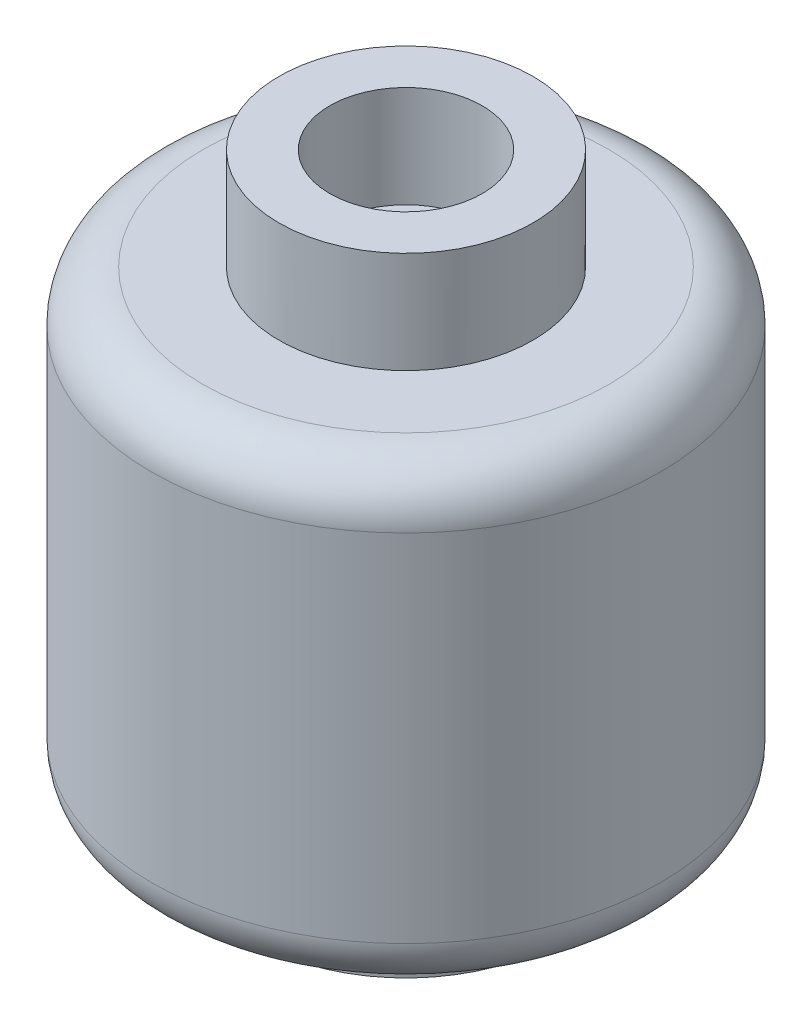
ISO-10303-21;
HEADER;
FILE_DESCRIPTION(('STEP AP214'),'2;1');
FILE_NAME('part.step','',(''),(''),'','','');
FILE_SCHEMA(('AUTOMOTIVE_DESIGN { 1 0 10303 214 1 1 1 1 }'));
ENDSEC;
DATA;
#1=APPLICATION_CONTEXT('core data for automotive mechanical design processes');
#2=APPLICATION_PROTOCOL_DEFINITION('international standard','automotive_design',2000,#1);
#3=PRODUCT_CONTEXT('',#1,'mechanical');
#4=PRODUCT('Part','Part','',(#3));
#5=PRODUCT_RELATED_PRODUCT_CATEGORY('part','',(#4));
#6=PRODUCT_DEFINITION_FORMATION('','',#4);
#7=PRODUCT_DEFINITION_CONTEXT('part definition',#1,'design');
#8=PRODUCT_DEFINITION('design','',#6,#7);
#9=PRODUCT_DEFINITION_SHAPE('','',#8);
#10=(LENGTH_UNIT() NAMED_UNIT(*) SI_UNIT(.MILLI.,.METRE.));
#11=(NAMED_UNIT(*) PLANE_ANGLE_UNIT() SI_UNIT($,.RADIAN.));
#12=(NAMED_UNIT(*) SI_UNIT($,.STERADIAN.) SOLID_ANGLE_UNIT());
#13=UNCERTAINTY_MEASURE_WITH_UNIT(LENGTH_MEASURE(1.E-05),#10,'distance_accuracy_value','');
#14=(GEOMETRIC_REPRESENTATION_CONTEXT(3) GLOBAL_UNCERTAINTY_ASSIGNED_CONTEXT((#13)) GLOBAL_UNIT_ASSIGNED_CONTEXT((#10,
#11,#12)) REPRESENTATION_CONTEXT('',''));
#15=CARTESIAN_POINT('',(0.,0.,0.));
#16=DIRECTION('',(0.,0.,1.));
#17=DIRECTION('',(1.,0.,0.));
#18=AXIS2_PLACEMENT_3D('',#15,#16,#17);
#19=CARTESIAN_POINT('',(0.,0.,0.));
#20=DIRECTION('',(0.,-1.,0.));
#21=DIRECTION('',(0.,0.,-1.));
#22=AXIS2_PLACEMENT_3D('',#19,#20,#21);
#23=CYLINDRICAL_SURFACE('',#22,5.);
#24=CARTESIAN_POINT('',(1.,6.20000000000001,-4.89897948556635));
#25=CARTESIAN_POINT('',(1.00000156872369,6.23586306138393,-4.89897950578697));
#26=CARTESIAN_POINT('',(1.00297865499742,6.27174942589603,-4.89837438780102));
#27=CARTESIAN_POINT('',(1.01480213788461,6.34252588569872,-4.89593828236374));
#28=CARTESIAN_POINT('',(1.02365483576842,6.37741486940713,-4.89410597880414));
#29=CARTESIAN_POINT('',(1.04694279696722,6.44516035531958,-4.88917697960863));
#30=CARTESIAN_POINT('',(1.06137459390475,6.47801810488525,-4.88608106900412));
#31=CARTESIAN_POINT('',(1.09535369815749,6.54079511555044,-4.87857576446154));
#32=CARTESIAN_POINT('',(1.11489983070227,6.57071504930283,-4.87416667213113));
#33=CARTESIAN_POINT('',(1.158584541537,6.62694759387382,-4.86396809819116));
#34=CARTESIAN_POINT('',(1.18274402944443,6.65324280362197,-4.8581722999757));
#35=CARTESIAN_POINT('',(1.23482548770339,6.70138615204387,-4.84519606525274));
#36=CARTESIAN_POINT('',(1.26274776156696,6.72323393162384,-4.83801551702904));
#37=CARTESIAN_POINT('',(1.3220159987903,6.76232468706743,-4.82216028574895));
#38=CARTESIAN_POINT('',(1.35341419297984,6.77947847351074,-4.81346121280438));
#39=CARTESIAN_POINT('',(1.41825919170025,6.80832243059168,-4.79475540886427));
#40=CARTESIAN_POINT('',(1.45170630441394,6.8200117770161,-4.78474848089322));
#41=CARTESIAN_POINT('',(1.52093621337638,6.83809739450905,-4.76320407601995));
#42=CARTESIAN_POINT('',(1.55675973455566,6.84428700126766,-4.75162434130285));
#43=CARTESIAN_POINT('',(1.6286066450515,6.85064895607429,-4.72748115596413));
#44=CARTESIAN_POINT('',(1.66463008196061,6.85081980390408,-4.71491746086553));
#45=CARTESIAN_POINT('',(1.73778614615725,6.8451409167464,-4.68846317663509));
#46=CARTESIAN_POINT('',(1.77488244422993,6.83898557672516,-4.67453760951146));
#47=CARTESIAN_POINT('',(1.84736298119408,6.82044202595814,-4.64637104142785));
#48=CARTESIAN_POINT('',(1.88274670164537,6.808051940576,-4.63212994682831));
#49=CARTESIAN_POINT('',(1.95230180183688,6.7767372104701,-4.60325879116952));
#50=CARTESIAN_POINT('',(1.9863675791089,6.75757032988729,-4.58863604916084));
#51=CARTESIAN_POINT('',(2.05076153491668,6.71324275804796,-4.56022117549695));
#52=CARTESIAN_POINT('',(2.08108914696987,6.68808116004063,-4.54642916989329));
#53=CARTESIAN_POINT('',(2.13666734384406,6.63263773864959,-4.52057310799027));
#54=CARTESIAN_POINT('',(2.16197848776713,6.60242630418322,-4.50848902040552));
#55=CARTESIAN_POINT('',(2.20700707163729,6.53735060646704,-4.48661882658691));
#56=CARTESIAN_POINT('',(2.22672828488387,6.50248950530907,-4.47683117099428));
#57=CARTESIAN_POINT('',(2.25819322579238,6.43227479843316,-4.46103664936299));
#58=CARTESIAN_POINT('',(2.27047667241963,6.39722069281157,-4.45477724754247));
#59=CARTESIAN_POINT('',(2.28891940690895,6.32514791726527,-4.44532990950916));
#60=CARTESIAN_POINT('',(2.29508397912362,6.28813097163815,-4.44213932309484));
#61=CARTESIAN_POINT('',(2.30064016771881,6.21728843643163,-4.43926371696131));
#62=CARTESIAN_POINT('',(2.30066024102716,6.18352384179948,-4.43925341767421));
#63=CARTESIAN_POINT('',(2.29549044487861,6.11650916532808,-4.44192887306966));
#64=CARTESIAN_POINT('',(2.29030144628595,6.08325899842914,-4.44461417709524));
#65=CARTESIAN_POINT('',(2.2751970896081,6.01922729119317,-4.4523641461491));
#66=CARTESIAN_POINT('',(2.26542901508946,5.98840154076483,-4.45735459869809));
#67=CARTESIAN_POINT('',(2.2416246503813,5.92887550666932,-4.4693730916337));
#68=CARTESIAN_POINT('',(2.22758750274041,5.90017565143361,-4.47640154134266));
#69=CARTESIAN_POINT('',(2.19475446312109,5.84381199746009,-4.49259464275087));
#70=CARTESIAN_POINT('',(2.17572169113451,5.81631645313862,-4.50186295811208));
#71=CARTESIAN_POINT('',(2.13398524683761,5.76484784883829,-4.52179628349611));
#72=CARTESIAN_POINT('',(2.11128006898282,5.74087624126394,-4.53246186600219));
#73=CARTESIAN_POINT('',(2.0603132664187,5.69458448372974,-4.55587219554798));
#74=CARTESIAN_POINT('',(2.03172164052999,5.67267848035175,-4.56871810401778));
#75=CARTESIAN_POINT('',(1.97152502592908,5.63395784409478,-4.59501563982341));
#76=CARTESIAN_POINT('',(1.93991878964557,5.61714533123995,-4.60846751670828));
#77=CARTESIAN_POINT('',(1.87189090526185,5.58784074539247,-4.63653729284295));
#78=CARTESIAN_POINT('',(1.83528586966668,5.57578175770425,-4.65116512383152));
#79=CARTESIAN_POINT('',(1.76037210083443,5.55828524067232,-4.68003221408688));
#80=CARTESIAN_POINT('',(1.72206312404718,5.55284866106503,-4.69427141733338));
#81=CARTESIAN_POINT('',(1.64430475631013,5.54884647842725,-4.72207434484025));
#82=CARTESIAN_POINT('',(1.60484715620024,5.55036544303433,-4.7356277187452));
#83=CARTESIAN_POINT('',(1.52645695557744,5.56062652830447,-4.76147365799019));
#84=CARTESIAN_POINT('',(1.48752423425738,5.5693669569861,-4.773766517909));
#85=CARTESIAN_POINT('',(1.41306705492273,5.59350921700795,-4.79632087238086));
#86=CARTESIAN_POINT('',(1.37746829085197,5.60862278292357,-4.80664505170919));
#87=CARTESIAN_POINT('',(1.30919735599651,5.64515691876416,-4.82568736070702));
#88=CARTESIAN_POINT('',(1.27652417332082,5.66657529692486,-4.83440604679051));
#89=CARTESIAN_POINT('',(1.2168920567295,5.71390195966075,-4.84974997525069));
#90=CARTESIAN_POINT('',(1.18972498577156,5.73952074592783,-4.85646016611695));
#91=CARTESIAN_POINT('',(1.14003765055289,5.79523971609589,-4.86836405127563));
#92=CARTESIAN_POINT('',(1.11751752335932,5.82534003213987,-4.87355770083774));
#93=CARTESIAN_POINT('',(1.07859052667666,5.88805669287335,-4.88231795370564));
#94=CARTESIAN_POINT('',(1.06200451295069,5.92055534099506,-4.88593312985496));
#95=CARTESIAN_POINT('',(1.0344876911731,5.98794797415707,-4.89183350906889));
#96=CARTESIAN_POINT('',(1.023550119189,6.02283903730369,-4.89412030326468));
#97=CARTESIAN_POINT('',(1.01042863815805,6.08161266137401,-4.89684186503736));
#98=CARTESIAN_POINT('',(1.00652375664101,6.10510902941916,-4.89764403406034));
#99=CARTESIAN_POINT('',(1.00130892684902,6.1524001773894,-4.89871283556499));
#100=CARTESIAN_POINT('',(0.999998958718624,6.17619495502974,-4.8989794721444));
#101=CARTESIAN_POINT('',(1.,6.20000000000001,-4.89897948556635));
#102=B_SPLINE_CURVE_WITH_KNOTS('',3,(#24,#25,#26,#27,#28,#29,#30,#31,#32,#33,#34,#35,#36,#37,
#38,#39,#40,#41,#42,#43,#44,#45,#46,#47,#48,#49,#50,#51,#52,#53,#54,#55,#56,#57,#58,#59,#60,#61,
#62,#63,#64,#65,#66,#67,#68,#69,#70,#71,#72,#73,#74,#75,#76,#77,#78,#79,#80,#81,#82,#83,#84,#85,
#86,#87,#88,#89,#90,#91,#92,#93,#94,#95,#96,#97,#98,#99,#100,#101),.UNSPECIFIED.,.T.,.F.,(4,2,2,
2,2,2,2,2,2,2,2,2,2,2,2,2,2,2,2,2,2,2,2,2,2,2,2,2,2,2,2,2,2,2,2,2,2,2,4),(0.,0.107502146017198,
0.215119768867601,0.322670634469891,0.43019681713439,0.538222445139969,0.6462567918788,
0.756220203332003,0.866200195455233,0.980156747892354,1.09414170460534,1.21390423220609,
1.33370279102324,1.45830794042833,1.58293194937669,1.70594505008929,1.82887491601095,
1.94124585538271,2.05351966485334,2.15430587581719,2.25507523992364,2.3528050697022,
2.45055454167926,2.55422921628436,2.65794650173261,2.77218412218085,2.88646922575167,
3.00956635425307,3.13268113435011,3.25729672894529,3.38188313451486,3.50135381061271,
3.6207830036443,3.73403554896939,3.84729143433638,3.95676250922337,4.06610218822255,
4.1374600953053,4.20881745637782),.UNSPECIFIED.);
#103=CARTESIAN_POINT('',(1.,6.20000000000001,-4.89897948556635));
#104=VERTEX_POINT('',#103);
#105=EDGE_CURVE('E74',#104,#104,#102,.T.);
#106=ORIENTED_EDGE('',*,*,#105,.F.);
#107=EDGE_LOOP('',(#106));
#108=FACE_BOUND('',#107,.T.);
#109=CARTESIAN_POINT('',(-2.3,6.2,-4.43959457608462));
#110=CARTESIAN_POINT('',(-2.29999812506802,6.23376367901104,-4.43959590662005));
#111=CARTESIAN_POINT('',(-2.29735527963792,6.26755114267601,-4.44096780412534));
#112=CARTESIAN_POINT('',(-2.28690648695137,6.3341211679552,-4.44635710752491));
#113=CARTESIAN_POINT('',(-2.27909442133407,6.36690249051653,-4.45037764836535));
#114=CARTESIAN_POINT('',(-2.25869913357096,6.43042247308173,-4.46076311262972));
#115=CARTESIAN_POINT('',(-2.24613138854528,6.46116738310239,-4.46712042923328));
#116=CARTESIAN_POINT('',(-2.21672094698416,6.52001627619411,-4.48178727121732));
#117=CARTESIAN_POINT('',(-2.19987807861373,6.54812015304884,-4.49009687506733));
#118=CARTESIAN_POINT('',(-2.16146430546663,6.60258307597295,-4.50871936393883));
#119=CARTESIAN_POINT('',(-2.13968914881422,6.62876912685022,-4.51911545385904));
#120=CARTESIAN_POINT('',(-2.09263608544451,6.6771942600584,-4.54109553218148));
#121=CARTESIAN_POINT('',(-2.06735681864845,6.69943180214097,-4.5526799813752));
#122=CARTESIAN_POINT('',(-2.01117236237794,6.74167522592829,-4.57779690806998));
#123=CARTESIAN_POINT('',(-1.97995632831079,6.76122203264447,-4.59140755455667));
#124=CARTESIAN_POINT('',(-1.91479516687287,6.79474970564269,-4.6189621878202));
#125=CARTESIAN_POINT('',(-1.8808489780272,6.80872839436278,-4.63290630275346));
#126=CARTESIAN_POINT('',(-1.80891617263393,6.83146833025578,-4.66148114234036));
#127=CARTESIAN_POINT('',(-1.77080935365711,6.83986364832348,-4.67610249687003));
#128=CARTESIAN_POINT('',(-1.69345543478325,6.84971654668912,-4.70466876542849));
#129=CARTESIAN_POINT('',(-1.65420831894334,6.85117402993979,-4.71861366999231));
#130=CARTESIAN_POINT('',(-1.57597436565614,6.84694985361812,-4.74531362816683));
#131=CARTESIAN_POINT('',(-1.53698753163237,6.84131556866086,-4.75807597249634));
#132=CARTESIAN_POINT('',(-1.46026544439222,6.82294082952768,-4.78217950617192));
#133=CARTESIAN_POINT('',(-1.42252982962489,6.81020244744065,-4.79352110873239));
#134=CARTESIAN_POINT('',(-1.35141826472214,6.77860919080583,-4.81403920055205));
#135=CARTESIAN_POINT('',(-1.3179195617974,6.76008169831667,-4.8232941306707));
#136=CARTESIAN_POINT('',(-1.25443098431052,6.71719555150431,-4.84019450796681));
#137=CARTESIAN_POINT('',(-1.22444010474567,6.69283857346974,-4.84784041663832));
#138=CARTESIAN_POINT('',(-1.1703996413989,6.64026821999595,-4.86116283805444));
#139=CARTESIAN_POINT('',(-1.14613384708423,6.61229632782405,-4.86691631700377));
#140=CARTESIAN_POINT('',(-1.10260925091337,6.55246437083802,-4.87696147784919));
#141=CARTESIAN_POINT('',(-1.08334962935697,6.5206049438176,-4.8812533990934));
#142=CARTESIAN_POINT('',(-1.05095875369573,6.45486363174064,-4.88832836599271));
#143=CARTESIAN_POINT('',(-1.03767282381066,6.42106198815578,-4.89114983844069));
#144=CARTESIAN_POINT('',(-1.0168991773021,6.35164312266193,-4.89551118022622));
#145=CARTESIAN_POINT('',(-1.00941105205768,6.31602602889187,-4.89705113988351));
#146=CARTESIAN_POINT('',(-1.00052599399766,6.24440378746397,-4.89887418995811));
#147=CARTESIAN_POINT('',(-0.999063698312998,6.20840707349181,-4.89917076809482));
#148=CARTESIAN_POINT('',(-1.00209674620955,6.13667654340366,-4.89855125681151));
#149=CARTESIAN_POINT('',(-1.00659192846425,6.10094272019503,-4.89763520022925));
#150=CARTESIAN_POINT('',(-1.02137894203311,6.03083740653594,-4.89457262804262));
#151=CARTESIAN_POINT('',(-1.03165734384401,5.99646295663634,-4.89242896292495));
#152=CARTESIAN_POINT('',(-1.0576725461085,5.92995718247656,-4.88687063433681));
#153=CARTESIAN_POINT('',(-1.07340928449704,5.89782583271577,-4.88345598531827));
#154=CARTESIAN_POINT('',(-1.10989933958094,5.83659142641726,-4.87529206174308));
#155=CARTESIAN_POINT('',(-1.13066931077326,5.80749889214164,-4.87053834768339));
#156=CARTESIAN_POINT('',(-1.17653144201685,5.75324569098518,-4.85966332997484));
#157=CARTESIAN_POINT('',(-1.20162370731765,5.72808511987762,-4.85354199302276));
#158=CARTESIAN_POINT('',(-1.25567798189552,5.68203622483806,-4.83984072339389));
#159=CARTESIAN_POINT('',(-1.28468462187544,5.66120550696568,-4.8322434424138));
#160=CARTESIAN_POINT('',(-1.34541503278201,5.62468788796898,-4.81568772478889));
#161=CARTESIAN_POINT('',(-1.37713909767426,5.6090015442413,-4.80672914079969));
#162=CARTESIAN_POINT('',(-1.44331517189571,5.58267858194895,-4.78728141776184));
#163=CARTESIAN_POINT('',(-1.47781951323458,5.57220093972653,-4.7767555385319));
#164=CARTESIAN_POINT('',(-1.54772794803604,5.55710011700076,-4.75456454632537));
#165=CARTESIAN_POINT('',(-1.58313224008343,5.55247824028405,-4.74289918026448));
#166=CARTESIAN_POINT('',(-1.65557732195721,5.54896631995416,-4.71811362760663));
#167=CARTESIAN_POINT('',(-1.6926170146506,5.5503551676754,-4.70495087491527));
#168=CARTESIAN_POINT('',(-1.76571140828362,5.55932234894575,-4.67801051902459));
#169=CARTESIAN_POINT('',(-1.80176582787881,5.56690243170286,-4.66423274310303));
#170=CARTESIAN_POINT('',(-1.87372731403228,5.58850604851756,-4.63580776547661));
#171=CARTESIAN_POINT('',(-1.90954229589548,5.60282446177242,-4.62115082194428));
#172=CARTESIAN_POINT('',(-1.97820531554219,5.63762702889237,-4.59217748603411));
#173=CARTESIAN_POINT('',(-2.01105262354813,5.65811269400359,-4.57786117805572));
#174=CARTESIAN_POINT('',(-2.0732244717038,5.7051088127454,-4.55004552514963));
#175=CARTESIAN_POINT('',(-2.10250284820064,5.73168753395944,-4.53655781952078));
#176=CARTESIAN_POINT('',(-2.1560901046185,5.79018972336251,-4.51133619308962));
#177=CARTESIAN_POINT('',(-2.18039937266147,5.82211277376767,-4.49960213533447));
#178=CARTESIAN_POINT('',(-2.22172826438218,5.88845238309648,-4.4793328811199));
#179=CARTESIAN_POINT('',(-2.2390976859563,5.92260450599742,-4.47064802319505));
#180=CARTESIAN_POINT('',(-2.26766152055505,5.99393686274579,-4.45622833058083));
#181=CARTESIAN_POINT('',(-2.27887023211448,6.03110985303888,-4.45048666706987));
#182=CARTESIAN_POINT('',(-2.29109776124512,6.09056742051539,-4.44419773201944));
#183=CARTESIAN_POINT('',(-2.29442856701929,6.11228002584481,-4.44247720641403));
#184=CARTESIAN_POINT('',(-2.29888023963348,6.15599172862197,-4.44017522460793));
#185=CARTESIAN_POINT('',(-2.300001222193,6.17799081100734,-4.43959370876191));
#186=CARTESIAN_POINT('',(-2.3,6.2,-4.43959457608462));
#187=B_SPLINE_CURVE_WITH_KNOTS('',3,(#109,#110,#111,#112,#113,#114,#115,#116,#117,#118,#119,
#120,#121,#122,#123,#124,#125,#126,#127,#128,#129,#130,#131,#132,#133,#134,#135,#136,#137,#138,
#139,#140,#141,#142,#143,#144,#145,#146,#147,#148,#149,#150,#151,#152,#153,#154,#155,#156,#157,
#158,#159,#160,#161,#162,#163,#164,#165,#166,#167,#168,#169,#170,#171,#172,#173,#174,#175,#176,
#177,#178,#179,#180,#181,#182,#183,#184,#185,#186),.UNSPECIFIED.,.T.,.F.,(4,2,2,2,2,2,2,2,2,2,2,
2,2,2,2,2,2,2,2,2,2,2,2,2,2,2,2,2,2,2,2,2,2,2,2,2,2,2,4),(0.,0.101204556162369,
0.202529114228452,0.303526713773192,0.40452837347427,0.510916737967762,0.617346512073878,
0.734633479254858,0.851966269723879,0.976382548008533,1.10080056663807,1.22439183858376,
1.34794708086105,1.46549698438377,1.58301312655323,1.69488360571627,1.80673575588673,
1.9154962801722,2.0242491384745,2.13181918581453,2.23938632025301,2.34670469249778,
2.45402184449863,2.56169906761254,2.66937891307903,2.77841072259549,2.8874543418872,
2.99964818476995,3.11186700323271,3.22934710116267,3.34686040219996,3.47007725828108,
3.59332433248496,3.71802633388025,3.84271859145621,3.95993123548691,4.07687067669987,
4.1428453251822,4.20881651874698),.UNSPECIFIED.);
#188=CARTESIAN_POINT('',(-2.3,6.2,-4.43959457608462));
#189=VERTEX_POINT('',#188);
#190=EDGE_CURVE('E84',#189,#189,#187,.T.);
#191=ORIENTED_EDGE('',*,*,#190,.F.);
#192=EDGE_LOOP('',(#191));
#193=FACE_BOUND('',#192,.T.);
#194=CARTESIAN_POINT('',(0.,8.99999999999999,0.));
#195=DIRECTION('',(0.,-1.,0.));
#196=DIRECTION('',(0.,0.,-1.));
#197=AXIS2_PLACEMENT_3D('',#194,#195,#196);
#198=CIRCLE('',#197,5.);
#199=CARTESIAN_POINT('',(0.,8.99999999999999,-5.));
#200=VERTEX_POINT('',#199);
#201=EDGE_CURVE('E141',#200,#200,#198,.T.);
#202=ORIENTED_EDGE('',*,*,#201,.T.);
#203=EDGE_LOOP('',(#202));
#204=FACE_BOUND('',#203,.T.);
#205=CARTESIAN_POINT('',(0.,2.00000000000001,0.));
#206=DIRECTION('',(0.,-1.,0.));
#207=DIRECTION('',(0.,0.,-1.));
#208=AXIS2_PLACEMENT_3D('',#205,#206,#207);
#209=CIRCLE('',#208,5.);
#210=CARTESIAN_POINT('',(0.,2.00000000000001,-5.));
#211=VERTEX_POINT('',#210);
#212=EDGE_CURVE('E149',#211,#211,#209,.T.);
#213=ORIENTED_EDGE('',*,*,#212,.F.);
#214=EDGE_LOOP('',(#213));
#215=FACE_BOUND('',#214,.T.);
#216=CARTESIAN_POINT('',(-2.1920310216783,3.30796897832171,-4.49388473372426));
#217=CARTESIAN_POINT('',(-2.19203989382054,3.31536049313591,-4.49387988155964));
#218=CARTESIAN_POINT('',(-2.19145216951387,3.32274502445388,-4.49416708637392));
#219=CARTESIAN_POINT('',(-2.1891546068307,3.33726856084877,-4.49528697229227));
#220=CARTESIAN_POINT('',(-2.18744882171491,3.34440835514677,-4.49611768302666));
#221=CARTESIAN_POINT('',(-2.18298660118061,3.35826307582907,-4.49828581107898));
#222=CARTESIAN_POINT('',(-2.18023077750409,3.36497824694372,-4.49962293336386));
#223=CARTESIAN_POINT('',(-2.17378026863328,3.37783109618784,-4.50274274527229));
#224=CARTESIAN_POINT('',(-2.17008498152936,3.38396840061333,-4.50452572053962));
#225=CARTESIAN_POINT('',(-2.16171016813163,3.39578311874742,-4.50855093565586));
#226=CARTESIAN_POINT('',(-2.15699559881476,3.40143006609363,-4.51080942207691));
#227=CARTESIAN_POINT('',(-2.14683728896301,3.4118597250654,-4.51565292338937));
#228=CARTESIAN_POINT('',(-2.14139334787007,3.41664219813053,-4.51823802808103));
#229=CARTESIAN_POINT('',(-2.1293736528847,3.42568934690085,-4.52391600578119));
#230=CARTESIAN_POINT('',(-2.12273944414948,3.42986069087341,-4.52703379636494));
#231=CARTESIAN_POINT('',(-2.10895287896103,3.43702905069902,-4.5334728165519));
#232=CARTESIAN_POINT('',(-2.10180022246091,3.44002537998886,-4.53679416378711));
#233=CARTESIAN_POINT('',(-2.08737980857593,3.44473030946788,-4.54344651338));
#234=CARTESIAN_POINT('',(-2.08012242134716,3.44647580810284,-4.54677405226762));
#235=CARTESIAN_POINT('',(-2.06544925264667,3.44880578897676,-4.55345866408099));
#236=CARTESIAN_POINT('',(-2.05803370616546,3.44939188683814,-4.55681568935138));
#237=CARTESIAN_POINT('',(-2.05060966544099,3.44939033455901,-4.56015350618814));
#238=B_SPLINE_CURVE_WITH_KNOTS('',3,(#216,#217,#218,#219,#220,#221,#222,#223,#224,#225,#226,
#227,#228,#229,#230,#231,#232,#233,#234,#235,#236,#237),.UNSPECIFIED.,.F.,.F.,(4,2,2,2,2,2,2,2,
2,2,4),(0.,0.0221347353454418,0.0441896670813337,0.0662317694314662,0.0882880297959428,
0.111277980951727,0.134274266763733,0.159470948812198,0.184682331468863,0.209115401679695,
0.233514400409308),.UNSPECIFIED.);
#239=CARTESIAN_POINT('',(-2.1920310216783,3.30796897832171,-4.49388473372426));
#240=VERTEX_POINT('',#239);
#241=CARTESIAN_POINT('',(-2.05060966544099,3.44939033455901,-4.56015350618814));
#242=VERTEX_POINT('',#241);
#243=EDGE_CURVE('E11',#240,#242,#238,.T.);
#244=ORIENTED_EDGE('',*,*,#243,.F.);
#245=CARTESIAN_POINT('',(2.1920310216783,3.3079689783217,-4.49388473372426));
#246=CARTESIAN_POINT('',(2.1329852864635,3.24894496168585,-4.52268309678667));
#247=CARTESIAN_POINT('',(2.07154515480206,3.1922576989043,-4.55121205387414));
#248=CARTESIAN_POINT('',(1.94394561125621,3.0837785042517,-4.60716301673319));
#249=CARTESIAN_POINT('',(1.87778329480569,3.03198963166128,-4.63458432467978));
#250=CARTESIAN_POINT('',(1.67169372276185,2.88387898486698,-4.71456634831918));
#251=CARTESIAN_POINT('',(1.52480314791688,2.79545604567751,-4.76452160426455));
#252=CARTESIAN_POINT('',(1.2927352314236,2.68107152816368,-4.83067294967581));
#253=CARTESIAN_POINT('',(1.21318555917039,2.64591269927123,-4.85130495688856));
#254=CARTESIAN_POINT('',(1.05070079070386,2.58218825332101,-4.88906560170676));
#255=CARTESIAN_POINT('',(0.967767715360954,2.55361876645564,-4.9061962948975));
#256=CARTESIAN_POINT('',(0.799329998591097,2.50353968216787,-4.93643372444016));
#257=CARTESIAN_POINT('',(0.713832762942422,2.48201155663858,-4.94955101538045));
#258=CARTESIAN_POINT('',(0.540779392934664,2.44625489027836,-4.97143423508457));
#259=CARTESIAN_POINT('',(0.453223560913794,2.43202528445903,-4.98020079869355));
#260=CARTESIAN_POINT('',(0.286215418164644,2.41221987097044,-4.99242757576322));
#261=CARTESIAN_POINT('',(0.206885775244561,2.40588779858419,-4.99635105538407));
#262=CARTESIAN_POINT('',(0.0478488113529438,2.39934745278175,-5.00040393265222));
#263=CARTESIAN_POINT('',(-0.0318586256786876,2.39914120213961,-5.00053207706263));
#264=CARTESIAN_POINT('',(-0.190941333540104,2.40486330227936,-4.99698562396111));
#265=CARTESIAN_POINT('',(-0.270316717077386,2.41078936715263,-4.99331244344755));
#266=CARTESIAN_POINT('',(-0.42813353299601,2.42867759931378,-4.98226609917856));
#267=CARTESIAN_POINT('',(-0.506574596563489,2.44064207432812,-4.97489152084916));
#268=CARTESIAN_POINT('',(-0.729365490467173,2.48341266576508,-4.94866544295479));
#269=CARTESIAN_POINT('',(-0.87187173641065,2.52156028962013,-4.92540727644533));
#270=CARTESIAN_POINT('',(-1.14824662936405,2.61677424409998,-4.86842354035322));
#271=CARTESIAN_POINT('',(-1.28210243431845,2.67386796387661,-4.83468282134871));
#272=CARTESIAN_POINT('',(-1.55672418721368,2.81419417283681,-4.75392497462917));
#273=CARTESIAN_POINT('',(-1.69585295554042,2.89996071192985,-4.70571286397488));
#274=CARTESIAN_POINT('',(-1.89175997525149,3.04281082736537,-4.62884236213235));
#275=CARTESIAN_POINT('',(-1.95486326006724,3.09272592874003,-4.60249444657428));
#276=CARTESIAN_POINT('',(-2.07672286483154,3.19703911436141,-4.54880673586574));
#277=CARTESIAN_POINT('',(-2.13548194933988,3.25143430015471,-4.52146758831769));
#278=CARTESIAN_POINT('',(-2.1920310216783,3.30796897832171,-4.49388473372426));
#279=B_SPLINE_CURVE_WITH_KNOTS('',3,(#245,#246,#247,#248,#249,#250,#251,#252,#253,#254,#255,
#256,#257,#258,#259,#260,#261,#262,#263,#264,#265,#266,#267,#268,#269,#270,#271,#272,#273,#274,
#275,#276,#277,#278),.UNSPECIFIED.,.F.,.F.,(4,2,2,2,2,2,2,2,2,2,2,2,2,2,2,2,4),(0.,
0.264776461874625,0.529717212320743,1.062456282023,1.33032388259535,1.59803376625972,
1.86503344257686,2.13199414763435,2.37071164214493,2.609507961376,2.84821529790668,
3.08701393145734,3.53292997565618,3.97949348085604,4.4882979422331,4.7420922917451,
4.99572371615684),.UNSPECIFIED.);
#280=CARTESIAN_POINT('',(2.1920310216783,3.3079689783217,-4.49388473372426));
#281=VERTEX_POINT('',#280);
#282=EDGE_CURVE('E57',#281,#240,#279,.T.);
#283=ORIENTED_EDGE('',*,*,#282,.F.);
#284=CARTESIAN_POINT('',(2.05060966544099,3.44939033455901,-4.56015350618814));
#285=CARTESIAN_POINT('',(2.05923284763423,3.44939336519703,-4.5562769754848));
#286=CARTESIAN_POINT('',(2.06784537903866,3.44860172797091,-4.55237357905702));
#287=CARTESIAN_POINT('',(2.08482793389469,3.44545937971092,-4.54462066877843));
#288=CARTESIAN_POINT('',(2.09319742268029,3.44310546845251,-4.54077128212568));
#289=CARTESIAN_POINT('',(2.10944461458457,3.43686550667467,-4.53324656602121));
#290=CARTESIAN_POINT('',(2.11732174139371,3.43297769824209,-4.5295714417142));
#291=CARTESIAN_POINT('',(2.13231407831919,3.42373514499219,-4.52253303184381));
#292=CARTESIAN_POINT('',(2.13942993299762,3.41838165504584,-4.51916948280145));
#293=CARTESIAN_POINT('',(2.15233736867419,3.40658173295129,-4.51303586917383));
#294=CARTESIAN_POINT('',(2.1581741059255,3.40019526312755,-4.51024592022444));
#295=CARTESIAN_POINT('',(2.16866257230676,3.38632057211198,-4.50521215797881));
#296=CARTESIAN_POINT('',(2.1733146478547,3.37883267401183,-4.50296818503718));
#297=CARTESIAN_POINT('',(2.18080561899281,3.36376168705353,-4.49934467692872));
#298=CARTESIAN_POINT('',(2.1837774491044,3.35625970453602,-4.49790201499438));
#299=CARTESIAN_POINT('',(2.18840823008973,3.34077843372877,-4.49565080849928));
#300=CARTESIAN_POINT('',(2.19007014886671,3.33280026875325,-4.49484083048628));
#301=CARTESIAN_POINT('',(2.19136621802226,3.32195134267023,-4.49420895894793));
#302=CARTESIAN_POINT('',(2.19161549706577,3.31916002299566,-4.49408739774615));
#303=CARTESIAN_POINT('',(2.19194768539087,3.3135692881472,-4.49392538738762));
#304=CARTESIAN_POINT('',(2.19203083944522,3.31076989097911,-4.49388481889422));
#305=CARTESIAN_POINT('',(2.1920310216783,3.3079689783217,-4.49388473372426));
#306=B_SPLINE_CURVE_WITH_KNOTS('',3,(#284,#285,#286,#287,#288,#289,#290,#291,#292,#293,#294,
#295,#296,#297,#298,#299,#300,#301,#302,#303,#304,#305),.UNSPECIFIED.,.F.,.F.,(4,2,2,2,2,2,2,2,
2,2,4),(0.,0.0283331818601552,0.0567245824169655,0.0851486157163481,0.113548388936371,
0.14067127065199,0.167786211981157,0.192246251852982,0.216650711320405,0.225061309739487,
0.233459506603712),.UNSPECIFIED.);
#307=CARTESIAN_POINT('',(2.05060966544099,3.44939033455901,-4.56015350618814));
#308=VERTEX_POINT('',#307);
#309=EDGE_CURVE('E72',#308,#281,#306,.T.);
#310=ORIENTED_EDGE('',*,*,#309,.F.);
#311=CARTESIAN_POINT('',(-2.05060966544099,3.44939033455901,-4.56015350618814));
#312=CARTESIAN_POINT('',(-1.99501648404705,3.39380960044506,-4.585153080676));
#313=CARTESIAN_POINT('',(-1.93715160924299,3.34045528985072,-4.60994968683317));
#314=CARTESIAN_POINT('',(-1.81701083184208,3.23842897001633,-4.65861354450834));
#315=CARTESIAN_POINT('',(-1.75473256880118,3.18975949972229,-4.68248028796378));
#316=CARTESIAN_POINT('',(-1.56098591464797,3.05079033342078,-4.75206906080866));
#317=CARTESIAN_POINT('',(-1.42311320220637,2.96803941140045,-4.79554283889403));
#318=CARTESIAN_POINT('',(-1.13266304568337,2.82542545005345,-4.87234255932021));
#319=CARTESIAN_POINT('',(-0.980031700194504,2.76565060424471,-4.90562930114495));
#320=CARTESIAN_POINT('',(-0.664934621115763,2.67250740191035,-4.95814717853788));
#321=CARTESIAN_POINT('',(-0.502497636795774,2.63906553596297,-4.97741743005368));
#322=CARTESIAN_POINT('',(-0.188752170027129,2.60225295119273,-4.99867439508794));
#323=CARTESIAN_POINT('',(-0.0378373062140034,2.59634565149173,-5.00211858240168));
#324=CARTESIAN_POINT('',(0.26278496233006,2.60801818398861,-4.99535102503718));
#325=CARTESIAN_POINT('',(0.41249234086434,2.62559852438444,-4.98513898488155));
#326=CARTESIAN_POINT('',(0.697397203660941,2.68157985150395,-4.9530808985569));
#327=CARTESIAN_POINT('',(0.832931516913035,2.71870523948753,-4.93194894684418));
#328=CARTESIAN_POINT('',(1.09576780839945,2.81136615093672,-4.88029437426417));
#329=CARTESIAN_POINT('',(1.22305926987222,2.86692466020052,-4.8497600322059));
#330=CARTESIAN_POINT('',(1.4764863881237,2.99960019774258,-4.7789755469934));
#331=CARTESIAN_POINT('',(1.60176186283587,3.07805805994749,-4.73815438478229));
#332=CARTESIAN_POINT('',(1.77861836471676,3.20830293551811,-4.67337858182355));
#333=CARTESIAN_POINT('',(1.83567061885963,3.25375360922665,-4.65122248047359));
#334=CARTESIAN_POINT('',(1.94599667867472,3.34863425863124,-4.60615255005856));
#335=CARTESIAN_POINT('',(1.99927221883448,3.39806238508573,-4.58323907600621));
#336=CARTESIAN_POINT('',(2.05060966544099,3.44939033455901,-4.56015350618814));
#337=B_SPLINE_CURVE_WITH_KNOTS('',3,(#311,#312,#313,#314,#315,#316,#317,#318,#319,#320,#321,
#322,#323,#324,#325,#326,#327,#328,#329,#330,#331,#332,#333,#334,#335,#336),.UNSPECIFIED.,.F.,
.F.,(4,2,2,2,2,2,2,2,2,2,2,2,4),(0.,0.247344986098241,0.494823274707448,0.99202556265293,
1.49111774024845,1.98881169619469,2.43960969263648,2.89041744307357,3.31490365378578,
3.73992119383987,4.19800075145766,4.4265345456294,4.65496269451142),.UNSPECIFIED.);
#338=EDGE_CURVE('E75',#242,#308,#337,.T.);
#339=ORIENTED_EDGE('',*,*,#338,.F.);
#340=EDGE_LOOP('',(#244,#283,#310,#339));
#341=FACE_BOUND('',#340,.T.);
#342=ADVANCED_FACE('F41',(#108,#193,#204,#215,#341),#23,.T.);
#343=ORIENTED_EDGE('',*,*,#282,.T.);
#344=ORIENTED_EDGE('',*,*,#243,.T.);
#345=ORIENTED_EDGE('',*,*,#338,.T.);
#346=ORIENTED_EDGE('',*,*,#309,.T.);
#347=EDGE_LOOP('',(#343,#344,#345,#346));
#348=FACE_BOUND('',#347,.T.);
#349=ADVANCED_FACE('F71',(#348),#23,.T.);
#350=ORIENTED_EDGE('',*,*,#105,.T.);
#351=EDGE_LOOP('',(#350));
#352=FACE_BOUND('',#351,.T.);
#353=ADVANCED_FACE('F203',(#352),#23,.T.);
#354=CARTESIAN_POINT('',(0.,10.,0.));
#355=DIRECTION('',(0.,-1.,0.));
#356=DIRECTION('',(0.,0.,-1.));
#357=AXIS2_PLACEMENT_3D('',#354,#355,#356);
#358=PLANE('',#357);
#359=CARTESIAN_POINT('',(0.,10.,0.));
#360=DIRECTION('',(0.,-1.,0.));
#361=DIRECTION('',(0.,0.,-1.));
#362=AXIS2_PLACEMENT_3D('',#359,#360,#361);
#363=CIRCLE('',#362,2.5);
#364=CARTESIAN_POINT('',(0.,10.,-2.5));
#365=VERTEX_POINT('',#364);
#366=EDGE_CURVE('E136',#365,#365,#363,.F.);
#367=ORIENTED_EDGE('',*,*,#366,.F.);
#368=EDGE_LOOP('',(#367));
#369=FACE_BOUND('',#368,.T.);
#370=CARTESIAN_POINT('',(0.,10.,0.));
#371=DIRECTION('',(0.,-1.,0.));
#372=DIRECTION('',(0.,0.,-1.));
#373=AXIS2_PLACEMENT_3D('',#370,#371,#372);
#374=CIRCLE('',#373,3.99999999999999);
#375=CARTESIAN_POINT('',(0.,10.,-3.99999999999999));
#376=VERTEX_POINT('',#375);
#377=EDGE_CURVE('E138',#376,#376,#374,.T.);
#378=ORIENTED_EDGE('',*,*,#377,.F.);
#379=EDGE_LOOP('',(#378));
#380=FACE_BOUND('',#379,.T.);
#381=ADVANCED_FACE('F215',(#369,#380),#358,.F.);
#382=CARTESIAN_POINT('',(0.,9.,0.));
#383=DIRECTION('',(0.,-1.,0.));
#384=DIRECTION('',(0.,0.,-1.));
#385=AXIS2_PLACEMENT_3D('',#382,#383,#384);
#386=TOROIDAL_SURFACE('',#385,4.,1.);
#387=ORIENTED_EDGE('',*,*,#201,.F.);
#388=EDGE_LOOP('',(#387));
#389=FACE_BOUND('',#388,.T.);
#390=ORIENTED_EDGE('',*,*,#377,.T.);
#391=EDGE_LOOP('',(#390));
#392=FACE_BOUND('',#391,.T.);
#393=ADVANCED_FACE('F101',(#389,#392),#386,.T.);
#394=ORIENTED_EDGE('',*,*,#190,.T.);
#395=EDGE_LOOP('',(#394));
#396=FACE_BOUND('',#395,.T.);
#397=ADVANCED_FACE('F96',(#396),#23,.T.);
#398=CARTESIAN_POINT('',(0.,2.,0.));
#399=DIRECTION('',(0.,-1.,0.));
#400=DIRECTION('',(0.,0.,-1.));
#401=AXIS2_PLACEMENT_3D('',#398,#399,#400);
#402=TOROIDAL_SURFACE('',#401,4.,0.999999999999999);
#403=CARTESIAN_POINT('',(0.,1.,0.));
#404=DIRECTION('',(0.,-1.,0.));
#405=DIRECTION('',(0.,0.,-1.));
#406=AXIS2_PLACEMENT_3D('',#403,#404,#405);
#407=CIRCLE('',#406,3.99999999999999);
#408=CARTESIAN_POINT('',(0.,1.,-3.99999999999999));
#409=VERTEX_POINT('',#408);
#410=EDGE_CURVE('E154',#409,#409,#407,.T.);
#411=ORIENTED_EDGE('',*,*,#410,.F.);
#412=EDGE_LOOP('',(#411));
#413=FACE_BOUND('',#412,.T.);
#414=ORIENTED_EDGE('',*,*,#212,.T.);
#415=EDGE_LOOP('',(#414));
#416=FACE_BOUND('',#415,.T.);
#417=ADVANCED_FACE('F105',(#413,#416),#402,.T.);
#418=CARTESIAN_POINT('',(-3.99999999999999,1.,0.));
#419=DIRECTION('',(0.,1.,0.));
#420=DIRECTION('',(0.,0.,1.));
#421=AXIS2_PLACEMENT_3D('',#418,#419,#420);
#422=PLANE('',#421);
#423=CARTESIAN_POINT('',(0.,1.,0.));
#424=DIRECTION('',(0.,-1.,0.));
#425=DIRECTION('',(0.,0.,-1.));
#426=AXIS2_PLACEMENT_3D('',#423,#424,#425);
#427=CIRCLE('',#426,3.);
#428=CARTESIAN_POINT('',(0.,1.,-3.));
#429=VERTEX_POINT('',#428);
#430=EDGE_CURVE('E153',#429,#429,#427,.T.);
#431=ORIENTED_EDGE('',*,*,#430,.F.);
#432=EDGE_LOOP('',(#431));
#433=FACE_BOUND('',#432,.T.);
#434=ORIENTED_EDGE('',*,*,#410,.T.);
#435=EDGE_LOOP('',(#434));
#436=FACE_BOUND('',#435,.T.);
#437=ADVANCED_FACE('F297',(#433,#436),#422,.F.);
#438=CARTESIAN_POINT('',(0.,0.,0.));
#439=DIRECTION('',(0.,-1.,0.));
#440=DIRECTION('',(0.,0.,-1.));
#441=AXIS2_PLACEMENT_3D('',#438,#439,#440);
#442=CYLINDRICAL_SURFACE('',#441,3.);
#443=CARTESIAN_POINT('',(0.,0.,0.));
#444=DIRECTION('',(0.,-1.,0.));
#445=DIRECTION('',(0.,0.,-1.));
#446=AXIS2_PLACEMENT_3D('',#443,#444,#445);
#447=CIRCLE('',#446,3.);
#448=CARTESIAN_POINT('',(0.,0.,-3.));
#449=VERTEX_POINT('',#448);
#450=EDGE_CURVE('E160',#449,#449,#447,.T.);
#451=ORIENTED_EDGE('',*,*,#450,.F.);
#452=EDGE_LOOP('',(#451));
#453=FACE_BOUND('',#452,.T.);
#454=ORIENTED_EDGE('',*,*,#430,.T.);
#455=EDGE_LOOP('',(#454));
#456=FACE_BOUND('',#455,.T.);
#457=ADVANCED_FACE('F289',(#453,#456),#442,.T.);
#458=CARTESIAN_POINT('',(-3.,0.,0.));
#459=DIRECTION('',(0.,1.,0.));
#460=DIRECTION('',(0.,0.,1.));
#461=AXIS2_PLACEMENT_3D('',#458,#459,#460);
#462=PLANE('',#461);
#463=CARTESIAN_POINT('',(0.,0.,0.));
#464=DIRECTION('',(0.,1.,0.));
#465=DIRECTION('',(0.,0.,1.));
#466=AXIS2_PLACEMENT_3D('',#463,#464,#465);
#467=CIRCLE('',#466,2.);
#468=CARTESIAN_POINT('',(0.,0.,2.));
#469=VERTEX_POINT('',#468);
#470=EDGE_CURVE('E163',#469,#469,#467,.F.);
#471=ORIENTED_EDGE('',*,*,#470,.F.);
#472=EDGE_LOOP('',(#471));
#473=FACE_BOUND('',#472,.T.);
#474=ORIENTED_EDGE('',*,*,#450,.T.);
#475=EDGE_LOOP('',(#474));
#476=FACE_BOUND('',#475,.T.);
#477=ADVANCED_FACE('F278',(#473,#476),#462,.F.);
#478=CARTESIAN_POINT('',(0.,9.,0.));
#479=DIRECTION('',(0.,-1.,0.));
#480=DIRECTION('',(0.,0.,-1.));
#481=AXIS2_PLACEMENT_3D('',#478,#479,#480);
#482=PLANE('',#481);
#483=CARTESIAN_POINT('',(0.,9.,0.));
#484=DIRECTION('',(0.,-1.,0.));
#485=DIRECTION('',(0.,0.,-1.));
#486=AXIS2_PLACEMENT_3D('',#483,#484,#485);
#487=CIRCLE('',#486,4.);
#488=CARTESIAN_POINT('',(0.,9.,-4.));
#489=VERTEX_POINT('',#488);
#490=EDGE_CURVE('E159',#489,#489,#487,.T.);
#491=ORIENTED_EDGE('',*,*,#490,.T.);
#492=EDGE_LOOP('',(#491));
#493=FACE_BOUND('',#492,.T.);
#494=ADVANCED_FACE('F269',(#493),#482,.T.);
#495=CARTESIAN_POINT('',(0.,0.,0.));
#496=DIRECTION('',(0.,-1.,0.));
#497=DIRECTION('',(0.,0.,-1.));
#498=AXIS2_PLACEMENT_3D('',#495,#496,#497);
#499=CYLINDRICAL_SURFACE('',#498,4.);
#500=CARTESIAN_POINT('',(0.,2.,0.));
#501=DIRECTION('',(0.,1.,0.));
#502=DIRECTION('',(0.,0.,1.));
#503=AXIS2_PLACEMENT_3D('',#500,#501,#502);
#504=CIRCLE('',#503,4.);
#505=CARTESIAN_POINT('',(0.,2.,4.));
#506=VERTEX_POINT('',#505);
#507=EDGE_CURVE('E166',#506,#506,#504,.F.);
#508=ORIENTED_EDGE('',*,*,#507,.T.);
#509=EDGE_LOOP('',(#508));
#510=FACE_BOUND('',#509,.T.);
#511=ORIENTED_EDGE('',*,*,#490,.F.);
#512=EDGE_LOOP('',(#511));
#513=FACE_BOUND('',#512,.T.);
#514=ADVANCED_FACE('F258',(#510,#513),#499,.F.);
#515=CARTESIAN_POINT('',(-3.99999999999999,2.,0.));
#516=DIRECTION('',(0.,1.,0.));
#517=DIRECTION('',(0.,0.,1.));
#518=AXIS2_PLACEMENT_3D('',#515,#516,#517);
#519=PLANE('',#518);
#520=CARTESIAN_POINT('',(0.,2.,0.));
#521=DIRECTION('',(0.,1.,0.));
#522=DIRECTION('',(0.,0.,1.));
#523=AXIS2_PLACEMENT_3D('',#520,#521,#522);
#524=CIRCLE('',#523,2.);
#525=CARTESIAN_POINT('',(0.,2.,2.));
#526=VERTEX_POINT('',#525);
#527=EDGE_CURVE('E165',#526,#526,#524,.F.);
#528=ORIENTED_EDGE('',*,*,#527,.T.);
#529=EDGE_LOOP('',(#528));
#530=FACE_BOUND('',#529,.T.);
#531=ORIENTED_EDGE('',*,*,#507,.F.);
#532=EDGE_LOOP('',(#531));
#533=FACE_BOUND('',#532,.T.);
#534=ADVANCED_FACE('F200',(#530,#533),#519,.T.);
#535=CARTESIAN_POINT('',(0.,0.,0.));
#536=DIRECTION('',(0.,-1.,0.));
#537=DIRECTION('',(0.,0.,-1.));
#538=AXIS2_PLACEMENT_3D('',#535,#536,#537);
#539=CYLINDRICAL_SURFACE('',#538,2.);
#540=ORIENTED_EDGE('',*,*,#470,.T.);
#541=EDGE_LOOP('',(#540));
#542=FACE_BOUND('',#541,.T.);
#543=ORIENTED_EDGE('',*,*,#527,.F.);
#544=EDGE_LOOP('',(#543));
#545=FACE_BOUND('',#544,.T.);
#546=ADVANCED_FACE('F189',(#542,#545),#539,.F.);
#547=CARTESIAN_POINT('',(0.,12.,0.));
#548=DIRECTION('',(0.,1.,0.));
#549=DIRECTION('',(0.,0.,1.));
#550=AXIS2_PLACEMENT_3D('',#547,#548,#549);
#551=PLANE('',#550);
#552=CARTESIAN_POINT('',(0.,12.,0.));
#553=DIRECTION('',(0.,1.,0.));
#554=DIRECTION('',(0.,0.,1.));
#555=AXIS2_PLACEMENT_3D('',#552,#553,#554);
#556=CIRCLE('',#555,2.5);
#557=CARTESIAN_POINT('',(0.,12.,2.5));
#558=VERTEX_POINT('',#557);
#559=EDGE_CURVE('E164',#558,#558,#556,.T.);
#560=ORIENTED_EDGE('',*,*,#559,.T.);
#561=EDGE_LOOP('',(#560));
#562=FACE_BOUND('',#561,.T.);
#563=CARTESIAN_POINT('',(0.,12.,0.));
#564=DIRECTION('',(0.,1.,0.));
#565=DIRECTION('',(0.,0.,1.));
#566=AXIS2_PLACEMENT_3D('',#563,#564,#565);
#567=CIRCLE('',#566,1.5);
#568=CARTESIAN_POINT('',(0.,12.,1.5));
#569=VERTEX_POINT('',#568);
#570=EDGE_CURVE('E174',#569,#569,#567,.T.);
#571=ORIENTED_EDGE('',*,*,#570,.F.);
#572=EDGE_LOOP('',(#571));
#573=FACE_BOUND('',#572,.T.);
#574=ADVANCED_FACE('F184',(#562,#573),#551,.T.);
#575=CARTESIAN_POINT('',(0.,12.,0.));
#576=DIRECTION('',(0.,-1.,0.));
#577=DIRECTION('',(0.,0.,-1.));
#578=AXIS2_PLACEMENT_3D('',#575,#576,#577);
#579=CYLINDRICAL_SURFACE('',#578,2.5);
#580=ORIENTED_EDGE('',*,*,#559,.F.);
#581=EDGE_LOOP('',(#580));
#582=FACE_BOUND('',#581,.T.);
#583=ORIENTED_EDGE('',*,*,#366,.T.);
#584=EDGE_LOOP('',(#583));
#585=FACE_BOUND('',#584,.T.);
#586=ADVANCED_FACE('F190',(#582,#585),#579,.T.);
#587=CARTESIAN_POINT('',(0.,12.,0.));
#588=DIRECTION('',(0.,-1.,0.));
#589=DIRECTION('',(0.,0.,-1.));
#590=AXIS2_PLACEMENT_3D('',#587,#588,#589);
#591=CYLINDRICAL_SURFACE('',#590,1.5);
#592=ORIENTED_EDGE('',*,*,#570,.T.);
#593=EDGE_LOOP('',(#592));
#594=FACE_BOUND('',#593,.T.);
#595=CARTESIAN_POINT('',(0.,10.,0.));
#596=DIRECTION('',(0.,1.,0.));
#597=DIRECTION('',(0.,0.,1.));
#598=AXIS2_PLACEMENT_3D('',#595,#596,#597);
#599=CIRCLE('',#598,1.5);
#600=CARTESIAN_POINT('',(0.,10.,1.5));
#601=VERTEX_POINT('',#600);
#602=EDGE_CURVE('E176',#601,#601,#599,.T.);
#603=ORIENTED_EDGE('',*,*,#602,.F.);
#604=EDGE_LOOP('',(#603));
#605=FACE_BOUND('',#604,.T.);
#606=ADVANCED_FACE('F185',(#594,#605),#591,.F.);
#607=ORIENTED_EDGE('',*,*,#602,.T.);
#608=EDGE_LOOP('',(#607));
#609=FACE_BOUND('',#608,.T.);
#610=ADVANCED_FACE('F216',(#609),#358,.F.);
#611=CLOSED_SHELL('',(#342,#349,#353,#381,#393,#397,#417,#437,#457,#477,#494,#514,#534,#546,
#574,#586,#606,#610));
#612=MANIFOLD_SOLID_BREP('B2',#611);
#613=ADVANCED_BREP_SHAPE_REPRESENTATION('',(#18,#612),#14);
#614=SHAPE_DEFINITION_REPRESENTATION(#9,#613);
ENDSEC;
END-ISO-10303-21;
